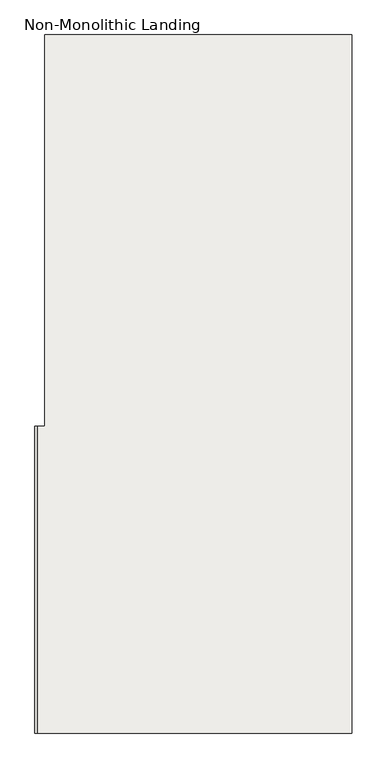
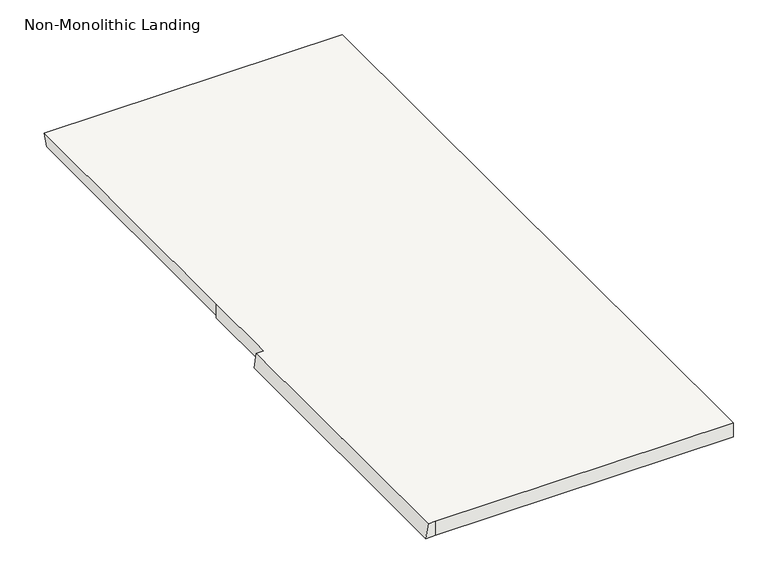
"""IFC4 building model written with IfcOpenShell, lengths in millimetres: slab geometry, Non-Monolithic Landing."""

from ifc_helpers import new_model, si_unit, origin, place, context, project, spatial, faceted_brep, source, transform, mapped, element, save


def non_monolithic_landing_122d3c1d(model_context):
    return source(origin(), model_context, "Body", "Brep", [
        faceted_brep([(-2716.9701746, -2816.1890637, 869.5652174), (-2724.1576746, -2816.1890637, 819.5652174), (-2724.1576746, -3816.2148449, 819.5652174), (-2716.9701746, -3816.2148449, 869.5652174), (-2691.9701746, -2541.1890637, 869.5652174), (-2691.9701746, -2816.1890637, 869.5652174), (-2691.9701746, -3816.2148449, 869.5652174), (-1691.9443934, -3816.2148449, 869.5652174), (-1691.9443934, -1541.1632824, 869.5652174), (-2691.9701746, -1541.1632824, 869.5652174), (-2691.9701746, -2816.1890637, 819.5652174), (-2691.9701746, -2541.1890637, 819.5652174), (-2684.7826746, -2541.1890637, 819.5652174), (-2684.7826746, -1541.1632824, 819.5652174), (-1691.9443934, -1541.1632824, 819.5652174), (-1691.9443934, -3816.2148449, 819.5652174), (-2691.9701746, -3816.2148449, 819.5652174)], [[[0, 1, 2, 3]], [[4, 5, 0, 3, 6, 7, 8, 9]], [[10, 11, 12, 13, 14, 15, 16, 2, 1]], [[5, 4, 11, 10]], [[0, 5, 10, 1]], [[6, 3, 2, 16]], [[7, 6, 16, 15]], [[8, 7, 15, 14]], [[9, 8, 14, 13]], [[4, 12, 11]], [[12, 4, 9, 13]]]),
    ])


if __name__ == "__main__":
    model = new_model("IFC4")
    model_context = context("Model", 3, world=origin())
    ifc_project = project(units=[si_unit("LENGTHUNIT", "METRE", prefix="MILLI")], contexts=[model_context])
    site = spatial("IfcSite", under=ifc_project)
    building = spatial("IfcBuilding", under=site)
    placement = place(None, origin())
    non_monolithic_landing_shape = non_monolithic_landing_122d3c1d(model_context)
    element("IfcSlab", 1, ObjectType="Non-Monolithic Landing", at=placement, inside=building, context=model_context, shape_type="MappedRepresentation", body=[
        mapped(non_monolithic_landing_shape, transform((0.0, 0.0, 0.0), x_axis=(1.0, 0.0, 0.0), y_axis=(0.0, 1.0, 0.0), z_axis=(0.0, 0.0, 1.0))),
    ])
    save(model, "model.ifc")
